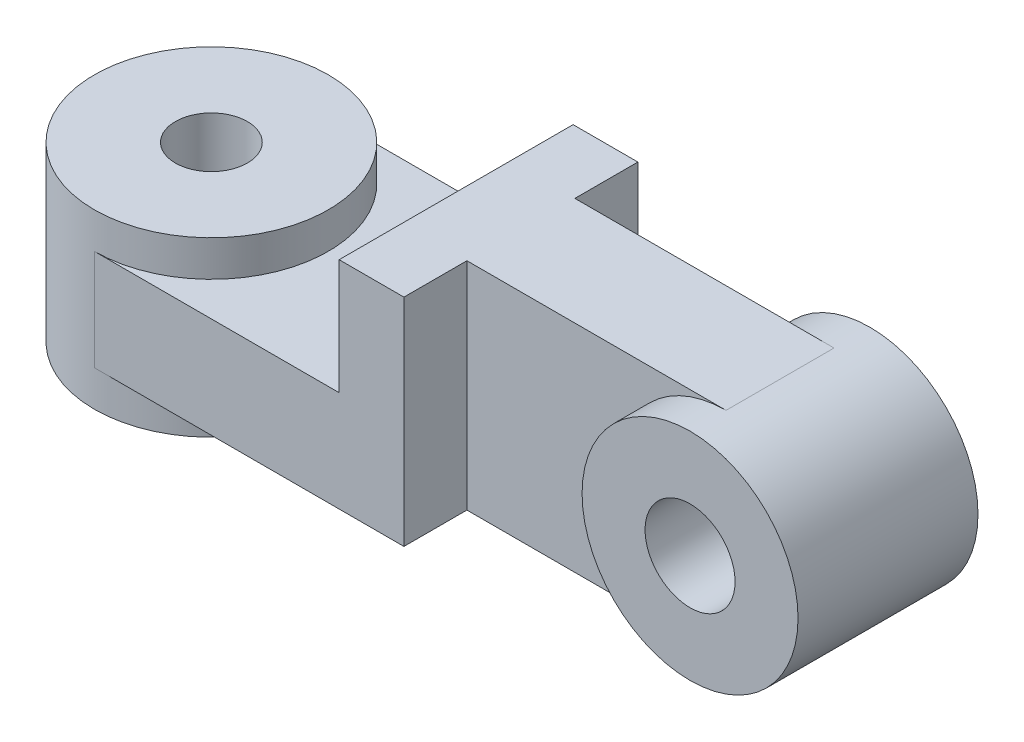
ISO-10303-21;
HEADER;
FILE_DESCRIPTION(('STEP AP214'),'2;1');
FILE_NAME('part.step','',(''),(''),'','','');
FILE_SCHEMA(('AUTOMOTIVE_DESIGN { 1 0 10303 214 1 1 1 1 }'));
ENDSEC;
DATA;
#1=APPLICATION_CONTEXT('core data for automotive mechanical design processes');
#2=APPLICATION_PROTOCOL_DEFINITION('international standard','automotive_design',2000,#1);
#3=PRODUCT_CONTEXT('',#1,'mechanical');
#4=PRODUCT('Part','Part','',(#3));
#5=PRODUCT_RELATED_PRODUCT_CATEGORY('part','',(#4));
#6=PRODUCT_DEFINITION_FORMATION('','',#4);
#7=PRODUCT_DEFINITION_CONTEXT('part definition',#1,'design');
#8=PRODUCT_DEFINITION('design','',#6,#7);
#9=PRODUCT_DEFINITION_SHAPE('','',#8);
#10=(LENGTH_UNIT() NAMED_UNIT(*) SI_UNIT(.MILLI.,.METRE.));
#11=(NAMED_UNIT(*) PLANE_ANGLE_UNIT() SI_UNIT($,.RADIAN.));
#12=(NAMED_UNIT(*) SI_UNIT($,.STERADIAN.) SOLID_ANGLE_UNIT());
#13=UNCERTAINTY_MEASURE_WITH_UNIT(LENGTH_MEASURE(1.E-05),#10,'distance_accuracy_value','');
#14=(GEOMETRIC_REPRESENTATION_CONTEXT(3) GLOBAL_UNCERTAINTY_ASSIGNED_CONTEXT((#13)) GLOBAL_UNIT_ASSIGNED_CONTEXT((#10,
#11,#12)) REPRESENTATION_CONTEXT('',''));
#15=CARTESIAN_POINT('',(0.,0.,0.));
#16=DIRECTION('',(0.,0.,1.));
#17=DIRECTION('',(1.,0.,0.));
#18=AXIS2_PLACEMENT_3D('',#15,#16,#17);
#19=CARTESIAN_POINT('',(68.,-28.,47.5));
#20=DIRECTION('',(0.,0.,1.));
#21=DIRECTION('',(1.,0.,0.));
#22=AXIS2_PLACEMENT_3D('',#19,#20,#21);
#23=PLANE('',#22);
#24=DIRECTION('',(1.,0.,0.));
#25=VECTOR('',#24,1.);
#26=CARTESIAN_POINT('',(68.,-28.,47.5));
#27=LINE('',#26,#25);
#28=CARTESIAN_POINT('',(68.,-28.,47.5));
#29=VERTEX_POINT('',#28);
#30=CARTESIAN_POINT('',(140.,-28.,47.5));
#31=VERTEX_POINT('',#30);
#32=EDGE_CURVE('E152',#29,#31,#27,.T.);
#33=ORIENTED_EDGE('',*,*,#32,.T.);
#34=CARTESIAN_POINT('',(140.,1.99999999999999,47.5));
#35=DIRECTION('',(0.,0.,1.));
#36=DIRECTION('',(1.,0.,0.));
#37=AXIS2_PLACEMENT_3D('',#34,#35,#36);
#38=CIRCLE('',#37,30.);
#39=CARTESIAN_POINT('',(140.,32.,47.5));
#40=VERTEX_POINT('',#39);
#41=EDGE_CURVE('E143',#40,#31,#38,.T.);
#42=ORIENTED_EDGE('',*,*,#41,.F.);
#43=DIRECTION('',(1.,0.,0.));
#44=VECTOR('',#43,1.);
#45=CARTESIAN_POINT('',(68.,32.,47.5));
#46=LINE('',#45,#44);
#47=CARTESIAN_POINT('',(68.,32.,47.5));
#48=VERTEX_POINT('',#47);
#49=EDGE_CURVE('E61',#48,#40,#46,.T.);
#50=ORIENTED_EDGE('',*,*,#49,.F.);
#51=DIRECTION('',(0.,1.,0.));
#52=VECTOR('',#51,1.);
#53=CARTESIAN_POINT('',(68.,-28.,47.5));
#54=LINE('',#53,#52);
#55=EDGE_CURVE('E175',#29,#48,#54,.T.);
#56=ORIENTED_EDGE('',*,*,#55,.F.);
#57=EDGE_LOOP('',(#33,#42,#50,#56));
#58=FACE_BOUND('',#57,.T.);
#59=ADVANCED_FACE('F50',(#58),#23,.T.);
#60=CARTESIAN_POINT('',(68.,0.,65.));
#61=DIRECTION('',(1.,0.,0.));
#62=DIRECTION('',(0.,0.,-1.));
#63=AXIS2_PLACEMENT_3D('',#60,#61,#62);
#64=PLANE('',#63);
#65=DIRECTION('',(0.,0.,-1.));
#66=VECTOR('',#65,1.);
#67=CARTESIAN_POINT('',(68.,-28.,65.));
#68=LINE('',#67,#66);
#69=CARTESIAN_POINT('',(68.,-28.,65.));
#70=VERTEX_POINT('',#69);
#71=EDGE_CURVE('E11',#70,#29,#68,.T.);
#72=ORIENTED_EDGE('',*,*,#71,.T.);
#73=ORIENTED_EDGE('',*,*,#55,.T.);
#74=DIRECTION('',(0.,0.,-1.));
#75=VECTOR('',#74,1.);
#76=CARTESIAN_POINT('',(68.,32.,65.));
#77=LINE('',#76,#75);
#78=CARTESIAN_POINT('',(68.,32.,65.));
#79=VERTEX_POINT('',#78);
#80=EDGE_CURVE('E139',#79,#48,#77,.T.);
#81=ORIENTED_EDGE('',*,*,#80,.F.);
#82=DIRECTION('',(0.,-1.,0.));
#83=VECTOR('',#82,1.);
#84=CARTESIAN_POINT('',(68.,0.,65.));
#85=LINE('',#84,#83);
#86=EDGE_CURVE('E202',#79,#70,#85,.T.);
#87=ORIENTED_EDGE('',*,*,#86,.T.);
#88=EDGE_LOOP('',(#72,#73,#81,#87));
#89=FACE_BOUND('',#88,.T.);
#90=ADVANCED_FACE('F242',(#89),#64,.T.);
#91=CARTESIAN_POINT('',(-18.,-48.,32.5));
#92=DIRECTION('',(0.,1.,0.));
#93=DIRECTION('',(0.,0.,1.));
#94=AXIS2_PLACEMENT_3D('',#91,#92,#93);
#95=CYLINDRICAL_SURFACE('',#94,32.5);
#96=CARTESIAN_POINT('',(-18.,10.,32.5));
#97=DIRECTION('',(0.,1.,0.));
#98=DIRECTION('',(0.,0.,1.));
#99=AXIS2_PLACEMENT_3D('',#96,#97,#98);
#100=CIRCLE('',#99,32.5);
#101=CARTESIAN_POINT('',(-18.,10.,65.));
#102=VERTEX_POINT('',#101);
#103=EDGE_CURVE('E184',#102,#102,#100,.T.);
#104=ORIENTED_EDGE('',*,*,#103,.F.);
#105=EDGE_LOOP('',(#104));
#106=FACE_BOUND('',#105,.T.);
#107=DIRECTION('',(0.,-1.,0.));
#108=VECTOR('',#107,1.);
#109=CARTESIAN_POINT('',(-18.,-28.,0.));
#110=LINE('',#109,#108);
#111=CARTESIAN_POINT('',(-18.,0.,0.));
#112=VERTEX_POINT('',#111);
#113=CARTESIAN_POINT('',(-18.,-28.,0.));
#114=VERTEX_POINT('',#113);
#115=EDGE_CURVE('E195',#112,#114,#110,.T.);
#116=ORIENTED_EDGE('',*,*,#115,.T.);
#117=CARTESIAN_POINT('',(-18.,-28.,32.5));
#118=DIRECTION('',(0.,-1.,0.));
#119=DIRECTION('',(0.,0.,-1.));
#120=AXIS2_PLACEMENT_3D('',#117,#118,#119);
#121=CIRCLE('',#120,32.5);
#122=CARTESIAN_POINT('',(-18.,-28.,65.));
#123=VERTEX_POINT('',#122);
#124=EDGE_CURVE('E189',#114,#123,#121,.T.);
#125=ORIENTED_EDGE('',*,*,#124,.T.);
#126=DIRECTION('',(0.,1.,0.));
#127=VECTOR('',#126,1.);
#128=CARTESIAN_POINT('',(-18.,0.,65.));
#129=LINE('',#128,#127);
#130=CARTESIAN_POINT('',(-18.,0.,65.));
#131=VERTEX_POINT('',#130);
#132=EDGE_CURVE('E197',#123,#131,#129,.T.);
#133=ORIENTED_EDGE('',*,*,#132,.T.);
#134=CARTESIAN_POINT('',(-18.,0.,32.5));
#135=DIRECTION('',(0.,1.,0.));
#136=DIRECTION('',(0.,0.,1.));
#137=AXIS2_PLACEMENT_3D('',#134,#135,#136);
#138=CIRCLE('',#137,32.5);
#139=EDGE_CURVE('E183',#131,#112,#138,.T.);
#140=ORIENTED_EDGE('',*,*,#139,.T.);
#141=EDGE_LOOP('',(#116,#125,#133,#140));
#142=FACE_BOUND('',#141,.T.);
#143=CARTESIAN_POINT('',(-18.,-38.,32.5));
#144=DIRECTION('',(0.,-1.,0.));
#145=DIRECTION('',(0.,0.,-1.));
#146=AXIS2_PLACEMENT_3D('',#143,#144,#145);
#147=CIRCLE('',#146,32.5);
#148=CARTESIAN_POINT('',(-18.,-38.,0.));
#149=VERTEX_POINT('',#148);
#150=EDGE_CURVE('E177',#149,#149,#147,.T.);
#151=ORIENTED_EDGE('',*,*,#150,.F.);
#152=EDGE_LOOP('',(#151));
#153=FACE_BOUND('',#152,.T.);
#154=ADVANCED_FACE('F248',(#106,#142,#153),#95,.T.);
#155=CARTESIAN_POINT('',(0.,-28.,65.));
#156=DIRECTION('',(0.,-1.,0.));
#157=DIRECTION('',(0.,0.,-1.));
#158=AXIS2_PLACEMENT_3D('',#155,#156,#157);
#159=PLANE('',#158);
#160=ORIENTED_EDGE('',*,*,#124,.F.);
#161=DIRECTION('',(-1.,0.,0.));
#162=VECTOR('',#161,1.);
#163=CARTESIAN_POINT('',(0.,-28.,0.));
#164=LINE('',#163,#162);
#165=CARTESIAN_POINT('',(68.,-28.,0.));
#166=VERTEX_POINT('',#165);
#167=EDGE_CURVE('E199',#166,#114,#164,.T.);
#168=ORIENTED_EDGE('',*,*,#167,.F.);
#169=CARTESIAN_POINT('',(68.,-28.,17.5));
#170=VERTEX_POINT('',#169);
#171=EDGE_CURVE('E54',#170,#166,#68,.T.);
#172=ORIENTED_EDGE('',*,*,#171,.F.);
#173=DIRECTION('',(-1.,0.,0.));
#174=VECTOR('',#173,1.);
#175=CARTESIAN_POINT('',(140.,-28.,17.5));
#176=LINE('',#175,#174);
#177=CARTESIAN_POINT('',(140.,-28.,17.5));
#178=VERTEX_POINT('',#177);
#179=EDGE_CURVE('E170',#178,#170,#176,.T.);
#180=ORIENTED_EDGE('',*,*,#179,.F.);
#181=DIRECTION('',(0.,0.,-1.));
#182=VECTOR('',#181,1.);
#183=CARTESIAN_POINT('',(140.,-28.,47.5));
#184=LINE('',#183,#182);
#185=EDGE_CURVE('E140',#31,#178,#184,.T.);
#186=ORIENTED_EDGE('',*,*,#185,.F.);
#187=ORIENTED_EDGE('',*,*,#32,.F.);
#188=ORIENTED_EDGE('',*,*,#71,.F.);
#189=DIRECTION('',(-1.,0.,0.));
#190=VECTOR('',#189,1.);
#191=CARTESIAN_POINT('',(0.,-28.,65.));
#192=LINE('',#191,#190);
#193=EDGE_CURVE('E196',#70,#123,#192,.T.);
#194=ORIENTED_EDGE('',*,*,#193,.T.);
#195=EDGE_LOOP('',(#160,#168,#172,#180,#186,#187,#188,#194));
#196=FACE_BOUND('',#195,.T.);
#197=ADVANCED_FACE('F47',(#196),#159,.T.);
#198=DIRECTION('',(0.,1.,0.));
#199=VECTOR('',#198,1.);
#200=CARTESIAN_POINT('',(68.,-28.,17.5));
#201=LINE('',#200,#199);
#202=CARTESIAN_POINT('',(68.,32.,17.5));
#203=VERTEX_POINT('',#202);
#204=EDGE_CURVE('E169',#170,#203,#201,.T.);
#205=ORIENTED_EDGE('',*,*,#204,.F.);
#206=ORIENTED_EDGE('',*,*,#171,.T.);
#207=DIRECTION('',(0.,-1.,0.));
#208=VECTOR('',#207,1.);
#209=CARTESIAN_POINT('',(68.,0.,0.));
#210=LINE('',#209,#208);
#211=CARTESIAN_POINT('',(68.,32.,0.));
#212=VERTEX_POINT('',#211);
#213=EDGE_CURVE('E215',#212,#166,#210,.T.);
#214=ORIENTED_EDGE('',*,*,#213,.F.);
#215=EDGE_CURVE('E228',#203,#212,#77,.T.);
#216=ORIENTED_EDGE('',*,*,#215,.F.);
#217=EDGE_LOOP('',(#205,#206,#214,#216));
#218=FACE_BOUND('',#217,.T.);
#219=ADVANCED_FACE('F233',(#218),#64,.T.);
#220=CARTESIAN_POINT('',(0.,32.,65.));
#221=DIRECTION('',(0.,1.,0.));
#222=DIRECTION('',(0.,0.,1.));
#223=AXIS2_PLACEMENT_3D('',#220,#221,#222);
#224=PLANE('',#223);
#225=DIRECTION('',(1.,0.,0.));
#226=VECTOR('',#225,1.);
#227=CARTESIAN_POINT('',(0.,32.,0.));
#228=LINE('',#227,#226);
#229=CARTESIAN_POINT('',(50.,32.,0.));
#230=VERTEX_POINT('',#229);
#231=EDGE_CURVE('E217',#230,#212,#228,.T.);
#232=ORIENTED_EDGE('',*,*,#231,.F.);
#233=DIRECTION('',(0.,0.,-1.));
#234=VECTOR('',#233,1.);
#235=CARTESIAN_POINT('',(50.,32.,65.));
#236=LINE('',#235,#234);
#237=CARTESIAN_POINT('',(50.,32.,65.));
#238=VERTEX_POINT('',#237);
#239=EDGE_CURVE('E223',#238,#230,#236,.T.);
#240=ORIENTED_EDGE('',*,*,#239,.F.);
#241=DIRECTION('',(1.,0.,0.));
#242=VECTOR('',#241,1.);
#243=CARTESIAN_POINT('',(0.,32.,65.));
#244=LINE('',#243,#242);
#245=EDGE_CURVE('E203',#238,#79,#244,.T.);
#246=ORIENTED_EDGE('',*,*,#245,.T.);
#247=ORIENTED_EDGE('',*,*,#80,.T.);
#248=ORIENTED_EDGE('',*,*,#49,.T.);
#249=DIRECTION('',(0.,0.,-1.));
#250=VECTOR('',#249,1.);
#251=CARTESIAN_POINT('',(140.,32.,32.5));
#252=LINE('',#251,#250);
#253=CARTESIAN_POINT('',(140.,32.,17.5));
#254=VERTEX_POINT('',#253);
#255=EDGE_CURVE('E133',#40,#254,#252,.T.);
#256=ORIENTED_EDGE('',*,*,#255,.T.);
#257=DIRECTION('',(-1.,0.,0.));
#258=VECTOR('',#257,1.);
#259=CARTESIAN_POINT('',(140.,32.,17.5));
#260=LINE('',#259,#258);
#261=EDGE_CURVE('E136',#254,#203,#260,.T.);
#262=ORIENTED_EDGE('',*,*,#261,.T.);
#263=ORIENTED_EDGE('',*,*,#215,.T.);
#264=EDGE_LOOP('',(#232,#240,#246,#247,#248,#256,#262,#263));
#265=FACE_BOUND('',#264,.T.);
#266=ADVANCED_FACE('F134',(#265),#224,.T.);
#267=CARTESIAN_POINT('',(50.,0.,65.));
#268=DIRECTION('',(-1.,0.,0.));
#269=DIRECTION('',(0.,0.,1.));
#270=AXIS2_PLACEMENT_3D('',#267,#268,#269);
#271=PLANE('',#270);
#272=DIRECTION('',(0.,1.,0.));
#273=VECTOR('',#272,1.);
#274=CARTESIAN_POINT('',(50.,0.,0.));
#275=LINE('',#274,#273);
#276=CARTESIAN_POINT('',(50.,0.,0.));
#277=VERTEX_POINT('',#276);
#278=EDGE_CURVE('E216',#277,#230,#275,.T.);
#279=ORIENTED_EDGE('',*,*,#278,.F.);
#280=DIRECTION('',(0.,0.,-1.));
#281=VECTOR('',#280,1.);
#282=CARTESIAN_POINT('',(50.,0.,65.));
#283=LINE('',#282,#281);
#284=CARTESIAN_POINT('',(50.,0.,65.));
#285=VERTEX_POINT('',#284);
#286=EDGE_CURVE('E72',#285,#277,#283,.T.);
#287=ORIENTED_EDGE('',*,*,#286,.F.);
#288=DIRECTION('',(0.,1.,0.));
#289=VECTOR('',#288,1.);
#290=CARTESIAN_POINT('',(50.,0.,65.));
#291=LINE('',#290,#289);
#292=EDGE_CURVE('E210',#285,#238,#291,.T.);
#293=ORIENTED_EDGE('',*,*,#292,.T.);
#294=ORIENTED_EDGE('',*,*,#239,.T.);
#295=EDGE_LOOP('',(#279,#287,#293,#294));
#296=FACE_BOUND('',#295,.T.);
#297=ADVANCED_FACE('F236',(#296),#271,.T.);
#298=CARTESIAN_POINT('',(0.,0.,65.));
#299=DIRECTION('',(0.,1.,0.));
#300=DIRECTION('',(0.,0.,1.));
#301=AXIS2_PLACEMENT_3D('',#298,#299,#300);
#302=PLANE('',#301);
#303=DIRECTION('',(1.,0.,0.));
#304=VECTOR('',#303,1.);
#305=CARTESIAN_POINT('',(0.,0.,0.));
#306=LINE('',#305,#304);
#307=EDGE_CURVE('E204',#112,#277,#306,.T.);
#308=ORIENTED_EDGE('',*,*,#307,.F.);
#309=ORIENTED_EDGE('',*,*,#139,.F.);
#310=DIRECTION('',(1.,0.,0.));
#311=VECTOR('',#310,1.);
#312=CARTESIAN_POINT('',(0.,0.,65.));
#313=LINE('',#312,#311);
#314=EDGE_CURVE('E209',#131,#285,#313,.T.);
#315=ORIENTED_EDGE('',*,*,#314,.T.);
#316=ORIENTED_EDGE('',*,*,#286,.T.);
#317=EDGE_LOOP('',(#308,#309,#315,#316));
#318=FACE_BOUND('',#317,.T.);
#319=ADVANCED_FACE('F255',(#318),#302,.T.);
#320=CARTESIAN_POINT('',(0.,0.,65.));
#321=DIRECTION('',(0.,0.,1.));
#322=DIRECTION('',(1.,0.,0.));
#323=AXIS2_PLACEMENT_3D('',#320,#321,#322);
#324=PLANE('',#323);
#325=ORIENTED_EDGE('',*,*,#314,.F.);
#326=ORIENTED_EDGE('',*,*,#132,.F.);
#327=ORIENTED_EDGE('',*,*,#193,.F.);
#328=ORIENTED_EDGE('',*,*,#86,.F.);
#329=ORIENTED_EDGE('',*,*,#245,.F.);
#330=ORIENTED_EDGE('',*,*,#292,.F.);
#331=EDGE_LOOP('',(#325,#326,#327,#328,#329,#330));
#332=FACE_BOUND('',#331,.T.);
#333=ADVANCED_FACE('F241',(#332),#324,.T.);
#334=CARTESIAN_POINT('',(0.,0.,0.));
#335=DIRECTION('',(0.,0.,1.));
#336=DIRECTION('',(1.,0.,0.));
#337=AXIS2_PLACEMENT_3D('',#334,#335,#336);
#338=PLANE('',#337);
#339=ORIENTED_EDGE('',*,*,#167,.T.);
#340=ORIENTED_EDGE('',*,*,#115,.F.);
#341=ORIENTED_EDGE('',*,*,#307,.T.);
#342=ORIENTED_EDGE('',*,*,#278,.T.);
#343=ORIENTED_EDGE('',*,*,#231,.T.);
#344=ORIENTED_EDGE('',*,*,#213,.T.);
#345=EDGE_LOOP('',(#339,#340,#341,#342,#343,#344));
#346=FACE_BOUND('',#345,.T.);
#347=ADVANCED_FACE('F232',(#346),#338,.F.);
#348=CARTESIAN_POINT('',(-18.,10.,32.5));
#349=DIRECTION('',(0.,1.,0.));
#350=DIRECTION('',(0.,0.,1.));
#351=AXIS2_PLACEMENT_3D('',#348,#349,#350);
#352=PLANE('',#351);
#353=CARTESIAN_POINT('',(-18.,10.,32.5));
#354=DIRECTION('',(0.,1.,0.));
#355=DIRECTION('',(0.,0.,1.));
#356=AXIS2_PLACEMENT_3D('',#353,#354,#355);
#357=CIRCLE('',#356,10.);
#358=CARTESIAN_POINT('',(-18.,10.,42.5));
#359=VERTEX_POINT('',#358);
#360=EDGE_CURVE('E172',#359,#359,#357,.T.);
#361=ORIENTED_EDGE('',*,*,#360,.F.);
#362=EDGE_LOOP('',(#361));
#363=FACE_BOUND('',#362,.T.);
#364=ORIENTED_EDGE('',*,*,#103,.T.);
#365=EDGE_LOOP('',(#364));
#366=FACE_BOUND('',#365,.T.);
#367=ADVANCED_FACE('F278',(#363,#366),#352,.T.);
#368=CARTESIAN_POINT('',(-18.,-38.,32.5));
#369=DIRECTION('',(0.,-1.,0.));
#370=DIRECTION('',(0.,0.,-1.));
#371=AXIS2_PLACEMENT_3D('',#368,#369,#370);
#372=PLANE('',#371);
#373=CARTESIAN_POINT('',(-18.,-38.,32.5));
#374=DIRECTION('',(0.,1.,0.));
#375=DIRECTION('',(0.,0.,1.));
#376=AXIS2_PLACEMENT_3D('',#373,#374,#375);
#377=CIRCLE('',#376,10.);
#378=CARTESIAN_POINT('',(-18.,-38.,42.5));
#379=VERTEX_POINT('',#378);
#380=EDGE_CURVE('E176',#379,#379,#377,.T.);
#381=ORIENTED_EDGE('',*,*,#380,.T.);
#382=EDGE_LOOP('',(#381));
#383=FACE_BOUND('',#382,.T.);
#384=ORIENTED_EDGE('',*,*,#150,.T.);
#385=EDGE_LOOP('',(#384));
#386=FACE_BOUND('',#385,.T.);
#387=ADVANCED_FACE('F273',(#383,#386),#372,.T.);
#388=CARTESIAN_POINT('',(-18.,-38.,32.5));
#389=DIRECTION('',(0.,1.,0.));
#390=DIRECTION('',(0.,0.,1.));
#391=AXIS2_PLACEMENT_3D('',#388,#389,#390);
#392=CYLINDRICAL_SURFACE('',#391,10.);
#393=ORIENTED_EDGE('',*,*,#380,.F.);
#394=EDGE_LOOP('',(#393));
#395=FACE_BOUND('',#394,.T.);
#396=ORIENTED_EDGE('',*,*,#360,.T.);
#397=EDGE_LOOP('',(#396));
#398=FACE_BOUND('',#397,.T.);
#399=ADVANCED_FACE('F275',(#395,#398),#392,.F.);
#400=CARTESIAN_POINT('',(140.,-28.,17.5));
#401=DIRECTION('',(0.,0.,-1.));
#402=DIRECTION('',(-1.,0.,0.));
#403=AXIS2_PLACEMENT_3D('',#400,#401,#402);
#404=PLANE('',#403);
#405=CARTESIAN_POINT('',(140.,1.99999999999999,17.5));
#406=DIRECTION('',(0.,0.,-1.));
#407=DIRECTION('',(-1.,0.,0.));
#408=AXIS2_PLACEMENT_3D('',#405,#406,#407);
#409=CIRCLE('',#408,30.);
#410=EDGE_CURVE('E146',#178,#254,#409,.T.);
#411=ORIENTED_EDGE('',*,*,#410,.F.);
#412=ORIENTED_EDGE('',*,*,#179,.T.);
#413=ORIENTED_EDGE('',*,*,#204,.T.);
#414=ORIENTED_EDGE('',*,*,#261,.F.);
#415=EDGE_LOOP('',(#411,#412,#413,#414));
#416=FACE_BOUND('',#415,.T.);
#417=ADVANCED_FACE('F250',(#416),#404,.T.);
#418=CARTESIAN_POINT('',(140.,1.99999999999999,7.5));
#419=DIRECTION('',(0.,0.,1.));
#420=DIRECTION('',(1.,0.,0.));
#421=AXIS2_PLACEMENT_3D('',#418,#419,#420);
#422=CYLINDRICAL_SURFACE('',#421,30.);
#423=CARTESIAN_POINT('',(140.,1.99999999999999,7.5));
#424=DIRECTION('',(0.,0.,1.));
#425=DIRECTION('',(1.,0.,0.));
#426=AXIS2_PLACEMENT_3D('',#423,#424,#425);
#427=CIRCLE('',#426,30.);
#428=CARTESIAN_POINT('',(170.,1.99999999999999,7.5));
#429=VERTEX_POINT('',#428);
#430=EDGE_CURVE('E157',#429,#429,#427,.T.);
#431=ORIENTED_EDGE('',*,*,#430,.T.);
#432=EDGE_LOOP('',(#431));
#433=FACE_BOUND('',#432,.T.);
#434=ORIENTED_EDGE('',*,*,#410,.T.);
#435=ORIENTED_EDGE('',*,*,#255,.F.);
#436=ORIENTED_EDGE('',*,*,#41,.T.);
#437=ORIENTED_EDGE('',*,*,#185,.T.);
#438=EDGE_LOOP('',(#434,#435,#436,#437));
#439=FACE_BOUND('',#438,.T.);
#440=CARTESIAN_POINT('',(140.,1.99999999999999,57.5));
#441=DIRECTION('',(0.,0.,1.));
#442=DIRECTION('',(1.,0.,0.));
#443=AXIS2_PLACEMENT_3D('',#440,#441,#442);
#444=CIRCLE('',#443,30.);
#445=CARTESIAN_POINT('',(170.,1.99999999999999,57.5));
#446=VERTEX_POINT('',#445);
#447=EDGE_CURVE('E155',#446,#446,#444,.T.);
#448=ORIENTED_EDGE('',*,*,#447,.F.);
#449=EDGE_LOOP('',(#448));
#450=FACE_BOUND('',#449,.T.);
#451=ADVANCED_FACE('F141',(#433,#439,#450),#422,.T.);
#452=CARTESIAN_POINT('',(140.,1.99999999999999,7.5));
#453=DIRECTION('',(0.,0.,1.));
#454=DIRECTION('',(1.,0.,0.));
#455=AXIS2_PLACEMENT_3D('',#452,#453,#454);
#456=PLANE('',#455);
#457=CARTESIAN_POINT('',(140.,1.99999999999999,7.5));
#458=DIRECTION('',(0.,0.,1.));
#459=DIRECTION('',(1.,0.,0.));
#460=AXIS2_PLACEMENT_3D('',#457,#458,#459);
#461=CIRCLE('',#460,12.5);
#462=CARTESIAN_POINT('',(152.5,1.99999999999999,7.5));
#463=VERTEX_POINT('',#462);
#464=EDGE_CURVE('E154',#463,#463,#461,.T.);
#465=ORIENTED_EDGE('',*,*,#464,.T.);
#466=EDGE_LOOP('',(#465));
#467=FACE_BOUND('',#466,.T.);
#468=ORIENTED_EDGE('',*,*,#430,.F.);
#469=EDGE_LOOP('',(#468));
#470=FACE_BOUND('',#469,.T.);
#471=ADVANCED_FACE('F304',(#467,#470),#456,.F.);
#472=CARTESIAN_POINT('',(140.,1.99999999999999,57.5));
#473=DIRECTION('',(0.,0.,1.));
#474=DIRECTION('',(1.,0.,0.));
#475=AXIS2_PLACEMENT_3D('',#472,#473,#474);
#476=PLANE('',#475);
#477=CARTESIAN_POINT('',(140.,1.99999999999999,57.5));
#478=DIRECTION('',(0.,0.,1.));
#479=DIRECTION('',(1.,0.,0.));
#480=AXIS2_PLACEMENT_3D('',#477,#478,#479);
#481=CIRCLE('',#480,12.5);
#482=CARTESIAN_POINT('',(152.5,1.99999999999999,57.5));
#483=VERTEX_POINT('',#482);
#484=EDGE_CURVE('E156',#483,#483,#481,.T.);
#485=ORIENTED_EDGE('',*,*,#484,.F.);
#486=EDGE_LOOP('',(#485));
#487=FACE_BOUND('',#486,.T.);
#488=ORIENTED_EDGE('',*,*,#447,.T.);
#489=EDGE_LOOP('',(#488));
#490=FACE_BOUND('',#489,.T.);
#491=ADVANCED_FACE('F315',(#487,#490),#476,.T.);
#492=CARTESIAN_POINT('',(140.,1.99999999999999,7.5));
#493=DIRECTION('',(0.,0.,1.));
#494=DIRECTION('',(1.,0.,0.));
#495=AXIS2_PLACEMENT_3D('',#492,#493,#494);
#496=CYLINDRICAL_SURFACE('',#495,12.5);
#497=ORIENTED_EDGE('',*,*,#464,.F.);
#498=EDGE_LOOP('',(#497));
#499=FACE_BOUND('',#498,.T.);
#500=ORIENTED_EDGE('',*,*,#484,.T.);
#501=EDGE_LOOP('',(#500));
#502=FACE_BOUND('',#501,.T.);
#503=ADVANCED_FACE('F320',(#499,#502),#496,.F.);
#504=CLOSED_SHELL('',(#59,#90,#154,#197,#219,#266,#297,#319,#333,#347,#367,#387,#399,#417,#451,
#471,#491,#503));
#505=MANIFOLD_SOLID_BREP('B2',#504);
#506=ADVANCED_BREP_SHAPE_REPRESENTATION('',(#18,#505),#14);
#507=SHAPE_DEFINITION_REPRESENTATION(#9,#506);
ENDSEC;
END-ISO-10303-21;
